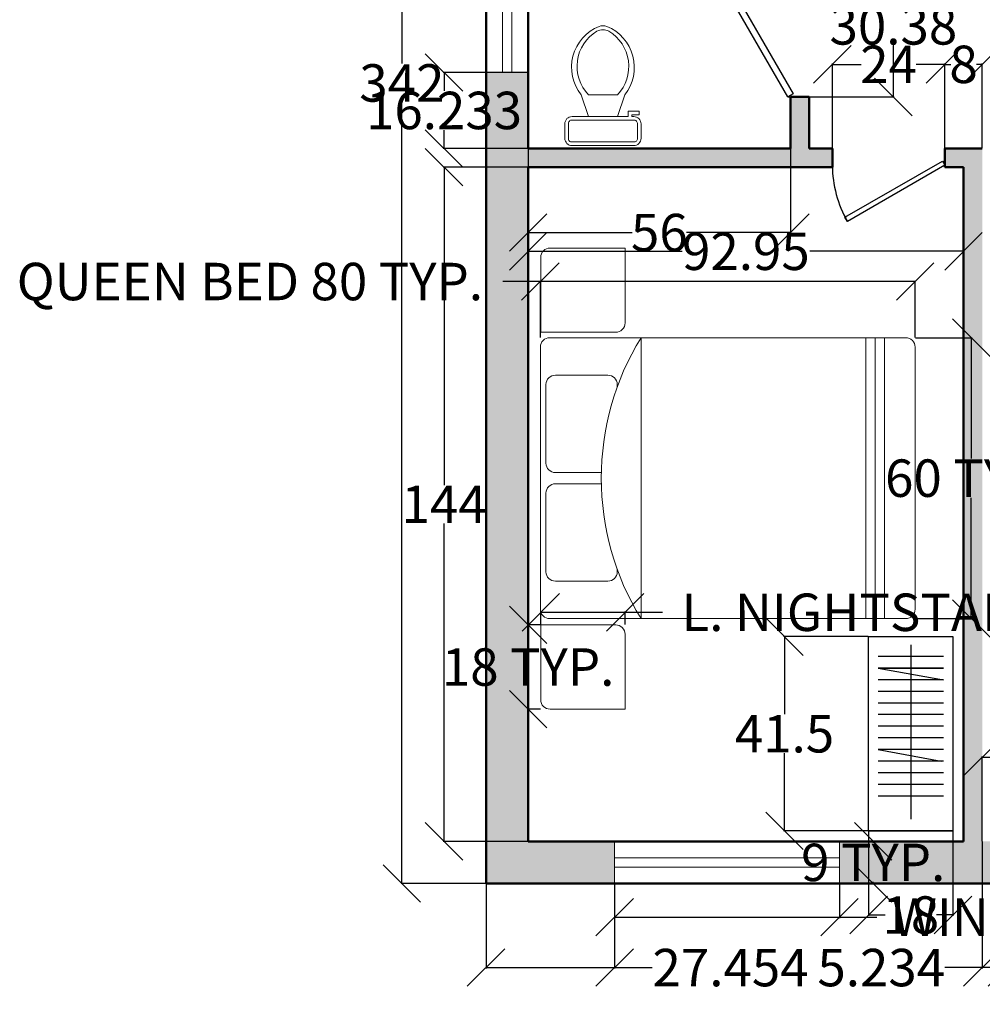
# Model space of a CAD drawing. Units: inches. Extents: x -87 to 308, y -349 to 42.
# Tile 1 of 6: x -87 to 119, y -349 to -139. Entities that reach past the tile are written whole.
import ezdxf

# ---------------------------------------------------------------- set-up
doc = ezdxf.new("R2010")
doc.units = ezdxf.units.IN
doc.header["$MEASUREMENT"] = 0
for name, color, linetype, lineweight in [('A-ANNO-DIMS', 2, 'Continuous', 18), ('A-DOOR', 3, 'Continuous', 25), ('A-FLOR-CASE', 9, 'Continuous', 25), ('A-FLOR-FIXT', 9, 'Continuous', 18), ('A-FURN', 8, 'Continuous', 18), ('A-GLAZ', 4, 'Continuous', 18), ('A-WALL', 7, 'Continuous', 50), ('A-WALL-PATT', 251, 'Continuous', 13)]:
    doc.layers.add(name, color=color, linetype=linetype, lineweight=lineweight)
doc.styles.get("Standard").update_dxf_attribs({"font": 'arial.ttf'})
doc.dimstyles.get("Standard").update_dxf_attribs({"dimtxt": 8, "dimasz": 8, "dimexe": 0.18, "dimexo": 0.0625, "dimgap": 0.09, "dimtad": 0, "dimtih": 1, "dimtoh": 1, "dimdec": 0, "dimzin": 0, "dimdsep": 46, "dimlunit": 4, "dimtxsty": 'Standard', "dimblk": 'OBLIQUE', "dimcen": 0.09, "dimadec": 0, "dimazin": 0, "dimtfac": 1, "dimtdec": 0, "dimtofl": 0, "dimtmove": 0, "dimatfit": 3, "dimldrblk": 'OBLIQUE', "dimfxl": 1, "dimtolj": 1, "dimtzin": 0, "dimarcsym": 0})

# ---------------------------------------------------------------- blocks, each defined once
blk = doc.blocks.new('*U6')
for p, q in [((-40, 0), (-40, 6)), ((0, 0), (0, 6))]:
    blk.add_line(p, q)
blk.add_lwpolyline([(0, 0), (-34.64, -20), (-35.52, -18.48), (-0.87, 1.52)], close=True)
blk.add_arc((0, 0), 40, 180, 210)
blk = doc.blocks.new('*U7')
for p, q in [((-40, 0), (-40, 6)), ((0, 0), (0, 6))]:
    blk.add_line(p, q)
blk.add_lwpolyline([(0, 0), (-34.64, -20), (-35.52, -18.48), (-0.88, 1.52)], close=True)
blk.add_arc((0, 0), 40, 180, 210)
blk = doc.blocks.new('Toilet - top')
for p, q in [((9.5, -6), (9.5, -2)), ((-8, -8.5), (-8, -8)), ((-7, -8), (-7, -9.5)), ((-4, -8), (-6, -14)), ((4, -8), (6, -14)), ((-10, -8.5), (-8, -8.5)), ((-10, -9.5), (-10, -8.5)), ((-7, -9.5), (-10, -9.5)), ((4, -14), (-4, -14))]:
    blk.add_line(p, q)
blk.add_lwpolyline([(-7, -8), (8.5, -8, 0.414214), (10.5, -6), (10.5, -2, 0.414214), (8.5, 0), (-8.5, 0, 0.414214), (-10.5, -2), (-10.5, -6, 0.414214), (-8.5, -8), (-8, -8)], format="xyb")
for points in [[(-9.5, -2), (-9.5, -6)], [(8.5, -1), (-8.5, -1)], [(-8.5, -7), (8.5, -7)]]:
    blk.add_lwpolyline(points)
for centre, radius, start, end in [((-8.62, -1.88), 0.884, 81.8699, 188.1301), ((8.62, -1.88), 0.884, 351.8699, 98.1301), ((-8.62, -6.12), 0.884, 171.8699, 278.1301), ((8.62, -6.12), 0.884, 261.8699, 8.1301), ((3.52, -21.58), 12.17, 141.4691, 247.9714), ((4.2, -21.82), 11.33, 136.3677, 238.9468), ((-3.52, -21.58), 12.17, 292.0284, 38.5307), ((-4.2, -21.82), 11.33, 301.053, 43.6321), ((0, -27.88), 4, 245.7318, 294.2682), ((0, -29), 4, 254.8605, 285.1395)]:
    blk.add_arc(centre, radius, start, end)
blk = doc.blocks.new('Bed - Queen')
for p, q in [((2, 0), (58, 0)), ((0, -78), (0, -2)), ((10, -1.2), (26.8, -1.2)), ((33.2, -1.2), (50, -1.2)), ((60, -2), (60, -78)), ((8, -14.4), (8, -3.2)), ((28.8, -3.2), (28.8, -13.02)), ((31.2, -13.02), (31.2, -3.2)), ((52, -3.2), (52, -14.4)), ((10.58, -16.4), (10, -16.4)), ((50, -16.4), (49.42, -16.4)), ((60, -21.5), (0, -21.5)), ((0, -69.5), (60, -69.5)), ((0, -71.5), (60, -71.5)), ((0, -73.5), (60, -73.5)), ((58, -80), (2, -80))]:
    blk.add_line(p, q)
for centre, radius, start, end in [((58, -2), 2, 0, 90), ((2, -2), 2, 90, 180), ((10, -3.2), 2, 90, 180), ((26.8, -3.2), 2, 0, 90), ((33.2, -3.2), 2, 90, 180), ((50, -3.2), 2, 0, 90), ((30, -70.21), 57.21, 58.3725, 121.6275), ((10, -14.4), 2, 180, 270), ((50, -14.4), 2, 270, 0), ((2, -78), 2, 180, 270), ((58, -78), 2, 270, 0)]:
    blk.add_arc(centre, radius, start, end)
blk = doc.blocks.new('WIN-48IN')
for p, q in [((0, 5.5), (48, 5.5)), ((0, 3.5), (48, 3.5))]:
    blk.add_line(p, q)
for points in [[(0, 0), (0, 9)], [(48, 9), (48, 0)]]:
    blk.add_lwpolyline(points)
blk = doc.blocks.new('WIN-24IN')
for p, q in [((0, 5.5), (24, 5.5)), ((0, 3.5), (24, 3.5))]:
    blk.add_line(p, q)
for points in [[(0, 0), (0, 9)], [(24, 9), (24, 0)]]:
    blk.add_lwpolyline(points)
blk = doc.blocks.new('NIGHTSTAND-18IN-L')
blk.add_lwpolyline([(2, 0), (18, 0), (18, 16, 0.414214), (16, 18), (0, 18), (0, 2, 0.414214)], format="xyb", close=True)
blk = doc.blocks.new('NIGHTSTAND-18IN-R')
blk.add_lwpolyline([(0, 0), (16, 0, 0.414214), (18, 2), (18, 18), (2, 18, 0.414214), (0, 16)], format="xyb", close=True)
blk = doc.blocks.new('_Oblique')
at = {"color": 0, "linetype": 'ByBlock', "lineweight": -2}
blk.add_line((-0.5, -0.5), (0.5, 0.5), dxfattribs=at)
blk = doc.blocks.new('*D23')
at = {"layer": 'A-ANNO-DIMS', "color": 0, "lineweight": -2, "transparency": 16777216}
for p, q in [((40.22, -323.73), (40.22, -331.05)), ((88.22, -323.73), (88.22, -331.05)), ((40.22, -330.87), (88.22, -330.87)), ((88.22, -330.87), (96.22, -330.87))]:
    blk.add_line(p, q, dxfattribs=at)
at = {"layer": 'Defpoints', "color": 0, "transparency": 16777216}
for p in [(40.22, -323.67), (88.22, -323.67), (88.22, -330.87)]:
    blk.add_point(p, dxfattribs=at)
at = {"layer": 'A-ANNO-DIMS', "color": 0, "lineweight": -2, "transparency": 16777216, "xscale": 8, "yscale": 8, "zscale": 8, "rotation": 180}
blk.add_blockref('_Oblique', (40.22, -330.87), dxfattribs=at)
at = {"layer": 'A-ANNO-DIMS', "color": 0, "lineweight": -2, "transparency": 16777216, "xscale": 8, "yscale": 8, "zscale": 8}
blk.add_blockref('_Oblique', (88.22, -330.87), dxfattribs=at)
at = {"layer": 'A-ANNO-DIMS', "color": 0, "transparency": 16777216, "insert": (142.01, -330.87), "char_height": 8, "attachment_point": 5}
blk.add_mtext('\\A1;WINDOW 48 TYP.', dxfattribs=at)
blk = doc.blocks.new('*D24')
at = {"layer": 'A-ANNO-DIMS', "color": 0, "lineweight": -2, "transparency": 16777216}
for p, q in [((88.28, -314.67), (95.6, -314.67)), ((95.42, -314.67), (95.42, -314.99)), ((88.28, -323.67), (95.6, -323.67)), ((95.42, -323.67), (95.42, -323.34))]:
    blk.add_line(p, q, dxfattribs=at)
at = {"layer": 'Defpoints', "color": 0, "transparency": 16777216}
for p in [(88.22, -314.67), (95.42, -314.67), (88.22, -323.67)]:
    blk.add_point(p, dxfattribs=at)
at = {"layer": 'A-ANNO-DIMS', "color": 0, "lineweight": -2, "transparency": 16777216, "xscale": 8, "yscale": 8, "zscale": 8}
for p, rotation in [((95.42, -314.67), 90), ((95.42, -323.67), 270)]:
    blk.add_blockref('_Oblique', p, dxfattribs=dict(at, rotation=rotation))
at = {"layer": 'A-ANNO-DIMS', "color": 0, "transparency": 16777216, "insert": (95.42, -319.17), "char_height": 8, "attachment_point": 5}
blk.add_mtext('\\A1;9 TYP.', dxfattribs=at)
blk = doc.blocks.new('*D29')
at = {"layer": 'A-ANNO-DIMS', "color": 0, "lineweight": -2, "transparency": 16777216}
for p, q in [((24.37, -195.09), (16.37, -195.09)), ((24.37, -207.03), (24.37, -194.91)), ((104.37, -195.09), (24.37, -195.09)), ((104.37, -207.03), (104.37, -194.91))]:
    blk.add_line(p, q, dxfattribs=at)
at = {"layer": 'Defpoints', "color": 0, "transparency": 16777216}
for p in [(24.37, -195.09), (24.37, -207.09), (104.37, -207.09)]:
    blk.add_point(p, dxfattribs=at)
at = {"layer": 'A-ANNO-DIMS', "color": 0, "lineweight": -2, "transparency": 16777216, "xscale": 8, "yscale": 8, "zscale": 8, "rotation": 180}
blk.add_blockref('_Oblique', (24.37, -195.09), dxfattribs=at)
at = {"layer": 'A-ANNO-DIMS', "color": 0, "lineweight": -2, "transparency": 16777216, "xscale": 8, "yscale": 8, "zscale": 8}
blk.add_blockref('_Oblique', (104.37, -195.09), dxfattribs=at)
at = {"layer": 'A-ANNO-DIMS', "color": 0, "transparency": 16777216, "insert": (-37.65, -195.09), "char_height": 8, "attachment_point": 5}
blk.add_mtext('\\A1;QUEEN BED 80 TYP.', dxfattribs=at)
blk = doc.blocks.new('*D30')
at = {"layer": 'A-ANNO-DIMS', "color": 0, "lineweight": -2, "transparency": 16777216}
for p, q in [((104.43, -207.09), (116.55, -207.09)), ((116.37, -207.09), (116.37, -232.92)), ((116.37, -267.09), (116.37, -241.27)), ((104.43, -267.09), (116.55, -267.09))]:
    blk.add_line(p, q, dxfattribs=at)
at = {"layer": 'Defpoints', "color": 0, "transparency": 16777216}
for p in [(104.37, -207.09), (116.37, -207.09), (104.37, -267.09)]:
    blk.add_point(p, dxfattribs=at)
at = {"layer": 'A-ANNO-DIMS', "color": 0, "lineweight": -2, "transparency": 16777216, "xscale": 8, "yscale": 8, "zscale": 8}
for p, rotation in [((116.37, -207.09), 90), ((116.37, -267.09), 270)]:
    blk.add_blockref('_Oblique', p, dxfattribs=dict(at, rotation=rotation))
at = {"layer": 'A-ANNO-DIMS', "color": 0, "transparency": 16777216, "insert": (116.37, -237.09), "char_height": 8, "attachment_point": 5}
blk.add_mtext('\\A1;60 TYP.', dxfattribs=at)
blk = doc.blocks.new('*D33')
at = {"layer": 'A-ANNO-DIMS', "color": 0, "lineweight": -2, "transparency": 16777216}
for p, q in [((26.45, -127.5), (26.45, -129.42)), ((38.45, -127.5), (38.45, -129.42)), ((26.45, -129.24), (38.45, -129.24)), ((38.45, -129.24), (46.45, -129.24))]:
    blk.add_line(p, q, dxfattribs=at)
at = {"layer": 'Defpoints', "color": 0, "transparency": 16777216}
for p in [(26.45, -127.44), (38.45, -127.44), (38.45, -129.24)]:
    blk.add_point(p, dxfattribs=at)
at = {"layer": 'A-ANNO-DIMS', "color": 0, "lineweight": -2, "transparency": 16777216, "xscale": 8, "yscale": 8, "zscale": 8, "rotation": 180}
blk.add_blockref('_Oblique', (26.45, -129.24), dxfattribs=at)
at = {"layer": 'A-ANNO-DIMS', "color": 0, "lineweight": -2, "transparency": 16777216, "xscale": 8, "yscale": 8, "zscale": 8}
blk.add_blockref('_Oblique', (38.45, -129.24), dxfattribs=at)
at = {"layer": 'A-ANNO-DIMS', "color": 0, "transparency": 16777216, "insert": (84.15, -129.24), "char_height": 8, "attachment_point": 5}
blk.add_mtext('\\A1;BASIN 12 TYP.', dxfattribs=at)
blk = doc.blocks.new('*D35')
at = {"layer": 'A-ANNO-DIMS', "color": 0, "lineweight": -2, "transparency": 16777216}
for p, q in [((24.45, -268.37), (24.45, -265.56)), ((24.45, -265.74), (42.45, -265.74)), ((42.45, -268.37), (42.45, -265.56)), ((42.45, -265.74), (50.45, -265.74))]:
    blk.add_line(p, q, dxfattribs=at)
at = {"layer": 'Defpoints', "color": 0, "transparency": 16777216}
for p in [(42.45, -265.74), (24.45, -268.44), (42.45, -268.44)]:
    blk.add_point(p, dxfattribs=at)
at = {"layer": 'A-ANNO-DIMS', "color": 0, "lineweight": -2, "transparency": 16777216, "xscale": 8, "yscale": 8, "zscale": 8, "rotation": 180}
blk.add_blockref('_Oblique', (24.45, -265.74), dxfattribs=at)
at = {"layer": 'A-ANNO-DIMS', "color": 0, "lineweight": -2, "transparency": 16777216, "xscale": 8, "yscale": 8, "zscale": 8}
blk.add_blockref('_Oblique', (42.45, -265.74), dxfattribs=at)
at = {"layer": 'A-ANNO-DIMS', "color": 0, "transparency": 16777216, "insert": (113.92, -265.74), "char_height": 8, "attachment_point": 5}
blk.add_mtext('\\A1;L. NIGHTSTAND 18 TYP.', dxfattribs=at)
blk = doc.blocks.new('*D36')
at = {"layer": 'A-ANNO-DIMS', "color": 0, "lineweight": -2, "transparency": 16777216}
for p, q in [((24.38, -268.44), (21.57, -268.44)), ((21.75, -268.44), (21.75, -273.26)), ((21.75, -286.44), (21.75, -281.61)), ((24.38, -286.44), (21.57, -286.44))]:
    blk.add_line(p, q, dxfattribs=at)
at = {"layer": 'Defpoints', "color": 0, "transparency": 16777216}
for p in [(21.75, -268.44), (24.45, -268.44), (24.45, -286.44)]:
    blk.add_point(p, dxfattribs=at)
at = {"layer": 'A-ANNO-DIMS', "color": 0, "lineweight": -2, "transparency": 16777216, "xscale": 8, "yscale": 8, "zscale": 8}
for p, rotation in [((21.75, -268.44), 90), ((21.75, -286.44), 270)]:
    blk.add_blockref('_Oblique', p, dxfattribs=dict(at, rotation=rotation))
at = {"layer": 'A-ANNO-DIMS', "color": 0, "transparency": 16777216, "insert": (21.75, -277.44), "char_height": 8, "attachment_point": 5}
blk.add_mtext('\\A1;18 TYP.', dxfattribs=at)
blk = doc.blocks.new('*D48')
at = {"layer": 'A-ANNO-DIMS', "color": 0, "lineweight": -2, "transparency": 16777216}
for p, q in [((12.7, 18.33), (-5.38, 18.33)), ((-5.2, 18.33), (-5.2, -148.49)), ((-5.2, -323.67), (-5.2, -156.85)), ((12.7, -323.67), (-5.38, -323.67))]:
    blk.add_line(p, q, dxfattribs=at)
at = {"layer": 'Defpoints', "color": 0, "transparency": 16777216}
for p in [(-5.2, 18.33), (12.76, 18.33), (12.76, -323.67)]:
    blk.add_point(p, dxfattribs=at)
at = {"layer": 'A-ANNO-DIMS', "color": 0, "lineweight": -2, "transparency": 16777216, "xscale": 8, "yscale": 8, "zscale": 8}
for p, rotation in [((-5.2, 18.33), 90), ((-5.2, -323.67), 270)]:
    blk.add_blockref('_Oblique', p, dxfattribs=dict(at, rotation=rotation))
at = {"layer": 'A-ANNO-DIMS', "color": 0, "transparency": 16777216, "insert": (-5.2, -152.67), "char_height": 8, "attachment_point": 5}
blk.add_mtext('\\A1;342', dxfattribs=at)
blk = doc.blocks.new('*D51')
at = {"layer": 'A-ANNO-DIMS', "color": 0, "lineweight": -2, "transparency": 16777216}
for p, q in [((12.76, -323.73), (12.76, -341.81)), ((40.22, -323.73), (40.22, -341.81)), ((12.76, -341.63), (40.22, -341.63)), ((40.22, -341.63), (48.22, -341.63))]:
    blk.add_line(p, q, dxfattribs=at)
at = {"layer": 'Defpoints', "color": 0, "transparency": 16777216}
for p in [(12.76, -323.67), (40.22, -323.67), (40.22, -341.63)]:
    blk.add_point(p, dxfattribs=at)
at = {"layer": 'A-ANNO-DIMS', "color": 0, "lineweight": -2, "transparency": 16777216, "xscale": 8, "yscale": 8, "zscale": 8, "rotation": 180}
blk.add_blockref('_Oblique', (12.76, -341.63), dxfattribs=at)
at = {"layer": 'A-ANNO-DIMS', "color": 0, "lineweight": -2, "transparency": 16777216, "xscale": 8, "yscale": 8, "zscale": 8}
blk.add_blockref('_Oblique', (40.22, -341.63), dxfattribs=at)
at = {"layer": 'A-ANNO-DIMS', "color": 0, "transparency": 16777216, "insert": (64.97, -341.63), "char_height": 8, "attachment_point": 5}
blk.add_mtext('\\A1;27.454', dxfattribs=at)
blk = doc.blocks.new('*D52')
at = {"layer": 'A-ANNO-DIMS', "color": 0, "lineweight": -2, "transparency": 16777216}
for p, q in [((118.71, -314.61), (118.71, -296.52)), ((142.71, -314.61), (142.71, -296.52)), ((118.71, -296.7), (124.84, -296.7)), ((142.71, -296.7), (136.58, -296.7))]:
    blk.add_line(p, q, dxfattribs=at)
at = {"layer": 'Defpoints', "color": 0, "transparency": 16777216}
for p in [(142.71, -296.7), (118.71, -314.67), (142.71, -314.67)]:
    blk.add_point(p, dxfattribs=at)
at = {"layer": 'A-ANNO-DIMS', "color": 0, "lineweight": -2, "transparency": 16777216, "xscale": 8, "yscale": 8, "zscale": 8, "rotation": 180}
blk.add_blockref('_Oblique', (118.71, -296.7), dxfattribs=at)
at = {"layer": 'A-ANNO-DIMS', "color": 0, "lineweight": -2, "transparency": 16777216, "xscale": 8, "yscale": 8, "zscale": 8}
blk.add_blockref('_Oblique', (142.71, -296.7), dxfattribs=at)
at = {"layer": 'A-ANNO-DIMS', "color": 0, "transparency": 16777216, "insert": (130.71, -296.7), "char_height": 8, "attachment_point": 5}
blk.add_mtext('\\A1;24', dxfattribs=at)
blk = doc.blocks.new('*D56')
at = {"layer": 'A-ANNO-DIMS', "color": 0, "lineweight": -2, "transparency": 16777216}
for p, q in [((21.7, -150.44), (3.62, -150.44)), ((3.8, -150.44), (3.8, -154.37)), ((3.8, -166.67), (3.8, -162.73)), ((21.7, -166.67), (3.62, -166.67))]:
    blk.add_line(p, q, dxfattribs=at)
at = {"layer": 'Defpoints', "color": 0, "transparency": 16777216}
for p in [(3.8, -150.44), (21.76, -150.44), (21.76, -166.67)]:
    blk.add_point(p, dxfattribs=at)
at = {"layer": 'A-ANNO-DIMS', "color": 0, "lineweight": -2, "transparency": 16777216, "xscale": 8, "yscale": 8, "zscale": 8}
for p, rotation in [((3.8, -150.44), 90), ((3.8, -166.67), 270)]:
    blk.add_blockref('_Oblique', p, dxfattribs=dict(at, rotation=rotation))
at = {"layer": 'A-ANNO-DIMS', "color": 0, "transparency": 16777216, "insert": (3.8, -158.55), "char_height": 8, "attachment_point": 5}
blk.add_mtext('\\A1;16.233', dxfattribs=at)
blk = doc.blocks.new('*D62')
at = {"layer": 'A-ANNO-DIMS', "color": 0, "lineweight": -2, "transparency": 16777216}
for p, q in [((21.76, -166.73), (21.76, -184.81)), ((77.76, -166.73), (77.76, -184.81)), ((21.76, -184.63), (43.95, -184.63)), ((77.76, -184.63), (55.58, -184.63))]:
    blk.add_line(p, q, dxfattribs=at)
at = {"layer": 'Defpoints', "color": 0, "transparency": 16777216}
for p in [(21.76, -166.67), (77.76, -166.67), (21.76, -184.63)]:
    blk.add_point(p, dxfattribs=at)
at = {"layer": 'A-ANNO-DIMS', "color": 0, "lineweight": -2, "transparency": 16777216, "xscale": 8, "yscale": 8, "zscale": 8, "rotation": 180}
blk.add_blockref('_Oblique', (21.76, -184.63), dxfattribs=at)
at = {"layer": 'A-ANNO-DIMS', "color": 0, "lineweight": -2, "transparency": 16777216, "xscale": 8, "yscale": 8, "zscale": 8}
blk.add_blockref('_Oblique', (77.76, -184.63), dxfattribs=at)
at = {"layer": 'A-ANNO-DIMS', "color": 0, "transparency": 16777216, "insert": (49.76, -184.63), "char_height": 8, "attachment_point": 5}
blk.add_mtext('\\A1;56', dxfattribs=at)
blk = doc.blocks.new('*D63')
at = {"layer": 'A-ANNO-DIMS', "color": 0, "lineweight": -2, "transparency": 16777216}
for p, q in [((21.76, -170.73), (21.76, -188.81)), ((114.71, -170.73), (114.71, -188.81)), ((21.76, -188.63), (54.62, -188.63)), ((114.71, -188.63), (81.86, -188.63))]:
    blk.add_line(p, q, dxfattribs=at)
at = {"layer": 'Defpoints', "color": 0, "transparency": 16777216}
for p in [(21.76, -170.67), (114.71, -170.67), (21.76, -188.63)]:
    blk.add_point(p, dxfattribs=at)
at = {"layer": 'A-ANNO-DIMS', "color": 0, "lineweight": -2, "transparency": 16777216, "xscale": 8, "yscale": 8, "zscale": 8, "rotation": 180}
blk.add_blockref('_Oblique', (21.76, -188.63), dxfattribs=at)
at = {"layer": 'A-ANNO-DIMS', "color": 0, "lineweight": -2, "transparency": 16777216, "xscale": 8, "yscale": 8, "zscale": 8}
blk.add_blockref('_Oblique', (114.71, -188.63), dxfattribs=at)
at = {"layer": 'A-ANNO-DIMS', "color": 0, "transparency": 16777216, "insert": (68.24, -188.63), "char_height": 8, "attachment_point": 5}
blk.add_mtext('\\A1;92.95', dxfattribs=at)
blk = doc.blocks.new('*D64')
at = {"layer": 'A-ANNO-DIMS', "color": 0, "lineweight": -2, "transparency": 16777216}
for p, q in [((21.7, -170.67), (3.62, -170.67)), ((3.8, -170.67), (3.8, -238.56)), ((3.8, -314.67), (3.8, -246.77)), ((21.7, -314.67), (3.62, -314.67))]:
    blk.add_line(p, q, dxfattribs=at)
at = {"layer": 'Defpoints', "color": 0, "transparency": 16777216}
for p in [(3.8, -170.67), (21.76, -170.67), (21.76, -314.67)]:
    blk.add_point(p, dxfattribs=at)
at = {"layer": 'A-ANNO-DIMS', "color": 0, "lineweight": -2, "transparency": 16777216, "xscale": 8, "yscale": 8, "zscale": 8}
for p, rotation in [((3.8, -170.67), 90), ((3.8, -314.67), 270)]:
    blk.add_blockref('_Oblique', p, dxfattribs=dict(at, rotation=rotation))
at = {"layer": 'A-ANNO-DIMS', "color": 0, "transparency": 16777216, "insert": (3.8, -242.67), "char_height": 8, "attachment_point": 5}
blk.add_mtext('\\A1;144', dxfattribs=at)
blk = doc.blocks.new('*D70')
at = {"layer": 'A-ANNO-DIMS', "color": 0, "lineweight": -2, "transparency": 16777216}
for p, q in [((81.83, -125.29), (99.91, -125.29)), ((99.73, -125.29), (99.73, -136.3)), ((99.73, -155.67), (99.73, -144.65)), ((81.83, -155.67), (99.91, -155.67))]:
    blk.add_line(p, q, dxfattribs=at)
at = {"layer": 'Defpoints', "color": 0, "transparency": 16777216}
for p in [(81.76, -125.29), (81.76, -155.67), (99.73, -155.67)]:
    blk.add_point(p, dxfattribs=at)
at = {"layer": 'A-ANNO-DIMS', "color": 0, "lineweight": -2, "transparency": 16777216, "xscale": 8, "yscale": 8, "zscale": 8}
for p, rotation in [((99.73, -125.29), 90), ((99.73, -155.67), 270)]:
    blk.add_blockref('_Oblique', p, dxfattribs=dict(at, rotation=rotation))
at = {"layer": 'A-ANNO-DIMS', "color": 0, "transparency": 16777216, "insert": (99.73, -140.48), "char_height": 8, "attachment_point": 5}
blk.add_mtext('\\A1;30.38', dxfattribs=at)
blk = doc.blocks.new('*D72')
at = {"layer": 'A-ANNO-DIMS', "color": 0, "lineweight": -2, "transparency": 16777216}
for p, q in [((86.71, -166.61), (86.71, -148.52)), ((86.71, -148.7), (92.84, -148.7)), ((110.71, -148.7), (104.58, -148.7)), ((110.71, -166.61), (110.71, -148.52))]:
    blk.add_line(p, q, dxfattribs=at)
at = {"layer": 'Defpoints', "color": 0, "transparency": 16777216}
for p in [(110.71, -148.7), (86.71, -166.67), (110.71, -166.67)]:
    blk.add_point(p, dxfattribs=at)
at = {"layer": 'A-ANNO-DIMS', "color": 0, "lineweight": -2, "transparency": 16777216, "xscale": 8, "yscale": 8, "zscale": 8, "rotation": 180}
blk.add_blockref('_Oblique', (86.71, -148.7), dxfattribs=at)
at = {"layer": 'A-ANNO-DIMS', "color": 0, "lineweight": -2, "transparency": 16777216, "xscale": 8, "yscale": 8, "zscale": 8}
blk.add_blockref('_Oblique', (110.71, -148.7), dxfattribs=at)
at = {"layer": 'A-ANNO-DIMS', "color": 0, "transparency": 16777216, "insert": (98.71, -148.7), "char_height": 8, "attachment_point": 5}
blk.add_mtext('\\A1;24', dxfattribs=at)
blk = doc.blocks.new('*D73')
at = {"layer": 'A-ANNO-DIMS', "color": 0, "lineweight": -2, "transparency": 16777216}
for p, q in [((110.71, -166.61), (110.71, -148.52)), ((110.71, -148.7), (111.99, -148.7)), ((118.71, -148.7), (117.44, -148.7)), ((118.71, -166.61), (118.71, -148.52))]:
    blk.add_line(p, q, dxfattribs=at)
at = {"layer": 'Defpoints', "color": 0, "transparency": 16777216}
for p in [(118.71, -148.7), (110.71, -166.67), (118.71, -166.67)]:
    blk.add_point(p, dxfattribs=at)
at = {"layer": 'A-ANNO-DIMS', "color": 0, "lineweight": -2, "transparency": 16777216, "xscale": 8, "yscale": 8, "zscale": 8, "rotation": 180}
blk.add_blockref('_Oblique', (110.71, -148.7), dxfattribs=at)
at = {"layer": 'A-ANNO-DIMS', "color": 0, "lineweight": -2, "transparency": 16777216, "xscale": 8, "yscale": 8, "zscale": 8}
blk.add_blockref('_Oblique', (118.71, -148.7), dxfattribs=at)
at = {"layer": 'A-ANNO-DIMS', "color": 0, "transparency": 16777216, "insert": (114.71, -148.7), "char_height": 8, "attachment_point": 5}
blk.add_mtext('\\A1;8', dxfattribs=at)
blk = doc.blocks.new('*D83')
at = {"layer": 'A-ANNO-DIMS', "color": 0, "lineweight": -2, "transparency": 16777216}
for p, q in [((94.38, -270.94), (76.3, -270.94)), ((76.48, -270.94), (76.48, -287.51)), ((76.48, -312.44), (76.48, -295.86)), ((94.38, -312.44), (76.3, -312.44))]:
    blk.add_line(p, q, dxfattribs=at)
at = {"layer": 'Defpoints', "color": 0, "transparency": 16777216}
for p in [(76.48, -270.94), (94.45, -270.94), (94.45, -312.44)]:
    blk.add_point(p, dxfattribs=at)
at = {"layer": 'A-ANNO-DIMS', "color": 0, "lineweight": -2, "transparency": 16777216, "xscale": 8, "yscale": 8, "zscale": 8}
for p, rotation in [((76.48, -270.94), 90), ((76.48, -312.44), 270)]:
    blk.add_blockref('_Oblique', p, dxfattribs=dict(at, rotation=rotation))
at = {"layer": 'A-ANNO-DIMS', "color": 0, "transparency": 16777216, "insert": (76.48, -291.69), "char_height": 8, "attachment_point": 5}
blk.add_mtext('\\A1;41.5', dxfattribs=at)
blk = doc.blocks.new('*D84')
at = {"layer": 'A-ANNO-DIMS', "color": 0, "lineweight": -2, "transparency": 16777216}
for p, q in [((94.45, -312.5), (94.45, -330.58)), ((112.45, -312.5), (112.45, -330.58)), ((94.45, -330.4), (97.99, -330.4)), ((112.45, -330.4), (108.9, -330.4))]:
    blk.add_line(p, q, dxfattribs=at)
at = {"layer": 'Defpoints', "color": 0, "transparency": 16777216}
for p in [(94.45, -312.44), (112.45, -312.44), (94.45, -330.4)]:
    blk.add_point(p, dxfattribs=at)
at = {"layer": 'A-ANNO-DIMS', "color": 0, "lineweight": -2, "transparency": 16777216, "xscale": 8, "yscale": 8, "zscale": 8, "rotation": 180}
blk.add_blockref('_Oblique', (94.45, -330.4), dxfattribs=at)
at = {"layer": 'A-ANNO-DIMS', "color": 0, "lineweight": -2, "transparency": 16777216, "xscale": 8, "yscale": 8, "zscale": 8}
blk.add_blockref('_Oblique', (112.45, -330.4), dxfattribs=at)
at = {"layer": 'A-ANNO-DIMS', "color": 0, "transparency": 16777216, "insert": (103.45, -330.4), "char_height": 8, "attachment_point": 5}
blk.add_mtext('\\A1;18', dxfattribs=at)
blk = doc.blocks.new('*D90')
at = {"layer": 'A-ANNO-DIMS', "color": 0, "lineweight": -2, "transparency": 16777216}
for p, q in [((123.95, -291), (123.95, -341.81)), ((118.71, -314.73), (118.71, -341.81)), ((118.71, -341.63), (110.71, -341.63)), ((123.95, -341.63), (118.71, -341.63))]:
    blk.add_line(p, q, dxfattribs=at)
at = {"layer": 'Defpoints', "color": 0, "transparency": 16777216}
for p in [(123.95, -290.94), (118.71, -314.67), (118.71, -341.63)]:
    blk.add_point(p, dxfattribs=at)
at = {"layer": 'A-ANNO-DIMS', "color": 0, "lineweight": -2, "transparency": 16777216, "xscale": 8, "yscale": 8, "zscale": 8, "rotation": 180}
blk.add_blockref('_Oblique', (118.71, -341.63), dxfattribs=at)
at = {"layer": 'A-ANNO-DIMS', "color": 0, "lineweight": -2, "transparency": 16777216, "xscale": 8, "yscale": 8, "zscale": 8}
blk.add_blockref('_Oblique', (123.95, -341.63), dxfattribs=at)
at = {"layer": 'A-ANNO-DIMS', "color": 0, "transparency": 16777216, "insert": (97.14, -341.63), "char_height": 8, "attachment_point": 5}
blk.add_mtext('\\A1;5.234', dxfattribs=at)

msp = doc.modelspace()

# ---------------------------------------------------------------- hatches: boundary and pattern name
at = {"layer": 'A-WALL-PATT'}
h = msp.add_hatch(color=256, dxfattribs=at)
h.dxf.hatch_style = 1
h.paths.add_polyline_path([(21.7637, -170.668), (86.7127, -170.668), (86.7127, -166.668), (81.7637, -166.668), (81.7637, -155.668), (77.7637, -155.668), (77.7637, -166.668), (21.7637, -166.668), (21.7637, -150.4351), (12.7637, -150.4351), (12.7637, -323.668), (40.2177, -323.668), (40.2177, -314.668), (21.7637, -314.668)])
h = msp.add_hatch(color=256, dxfattribs=at)
h.dxf.hatch_style = 1
h.paths.add_polyline_path([(118.7127, -170.668), (118.7127, -166.668), (114.7127, -166.668), (110.7127, -166.668), (110.7127, -170.668), (114.7127, -170.668), (114.7127, -314.668), (88.2177, -314.668), (88.2177, -323.668), (142.7127, -323.668), (142.7127, -319.1107), (142.7127, -314.668), (118.7127, -314.668)])

# ---------------------------------------------------------------- linework, layer by layer
at = {"layer": 'A-FLOR-CASE'}
for p, q in [((94.4465, -270.9351), (112.4465, -270.9351)), ((103.4465, -272.711), (103.4465, -309.9524)), ((110.4465, -275.1937), (96.4465, -275.1937)), ((110.4465, -282.642), (96.4465, -282.642)), ((110.4465, -285.1248), (96.4465, -285.1248)), ((110.4465, -287.6075), (96.4465, -287.6075)), ((110.4465, -290.0903), (96.4465, -290.0903)), ((110.4465, -292.573), (96.4465, -292.573)), ((110.4465, -297.5386), (96.4465, -297.5386)), ((110.4465, -300.0213), (96.4465, -300.0213)), ((110.4465, -302.5041), (96.4465, -302.5041)), ((110.4465, -304.9868), (96.4465, -304.9868))]:
    msp.add_line(p, q, dxfattribs=at)
for points in [[(94.4465, -312.4351), (94.4465, -270.9351)], [(112.4465, -270.9351), (112.4465, -312.4351), (94.4465, -312.4351), (112.4465, -312.4351)], [(96.4465, -277.6765), (110.4465, -277.6765), (96.4465, -277.6765), (110.4465, -280.1593), (96.4465, -280.1593)], [(110.4465, -295.0558), (96.4465, -295.0558), (109.9465, -297.5386)]]:
    msp.add_lwpolyline(points, dxfattribs=at)
at = {"layer": 'A-WALL'}
for p, q in [((21.7637, -166.668), (21.7637, -114.668)), ((77.7637, -166.668), (77.7637, -155.668)), ((81.7637, -155.668), (77.7637, -155.668)), ((81.7637, -166.668), (81.7637, -155.668)), ((77.7637, -166.668), (21.7637, -166.668)), ((86.7127, -166.668), (81.7637, -166.668)), ((86.7127, -170.668), (86.7127, -166.668)), ((114.7127, -166.668), (110.7127, -166.668)), ((110.7127, -170.668), (110.7127, -166.668)), ((114.7127, -166.668), (118.7127, -166.668)), ((21.7637, -314.668), (21.7637, -170.668)), ((86.7127, -170.668), (21.7637, -170.668)), ((114.7127, -170.668), (110.7127, -170.668)), ((114.7127, -170.668), (114.7127, -314.668)), ((114.7127, -314.668), (21.7637, -314.668))]:
    msp.add_line(p, q, dxfattribs=at)
msp.add_lwpolyline([(142.7127, -323.668), (12.7637, -323.668), (12.7637, 18.332), (246.7637, 18.332), (246.7637, -323.668), (172.7127, -323.668)], dxfattribs=at)

# ---------------------------------------------------------------- block references
at = {"layer": 'A-DOOR', "xscale": 0.7595575434647344, "yscale": 0.7595575434647344, "zscale": 0.7595575434647344, "rotation": 270}
msp.add_blockref('*U6', (77.2063, -155.668), dxfattribs=at)
at = {"layer": 'A-DOOR', "xscale": 0.6, "yscale": 0.6, "zscale": 0.6}
msp.add_blockref('*U7', (110.7127, -170.268), dxfattribs=at)
at = {"layer": 'A-FLOR-FIXT', "xscale": 0.7748713842371889, "yscale": 0.7748713842371889, "zscale": 0.7748713842371889, "rotation": 180}
msp.add_blockref('Toilet - top', (37.7161, -166.0445), dxfattribs=at)
at = {"layer": 'A-FURN'}
for name, p in [('NIGHTSTAND-18IN-R', (24.447, -205.935)), ('NIGHTSTAND-18IN-L', (24.447, -286.435))]:
    msp.add_blockref(name, p, dxfattribs=at)
at = {"layer": 'A-FURN', "rotation": 90}
msp.add_blockref('Bed - Queen', (24.3666, -267.0911), dxfattribs=at)
at = {"layer": 'A-GLAZ', "rotation": 270}
msp.add_blockref('WIN-24IN', (12.7637, -126.4351), dxfattribs=at)
at = {"layer": 'A-GLAZ'}
msp.add_blockref('WIN-48IN', (40.2176, -323.668), dxfattribs=at)

# ---------------------------------------------------------------- dimensions: what is measured, and where the dimension line sits
at = {"layer": 'A-ANNO-DIMS'}
for base, p1, p2, angle, override, picture, middle in [((-5.2008, 18.332), (12.7637, -323.668), (12.7637, 18.332), 90, {"dimdec": 0, "dimlfac": 1, "dimrnd": 0, "dimzin": 0, "dimdsep": 46, "dimlunit": 2}, '*D48', (-5.2008, -152.668)), ((99.7282, -155.668), (81.7637, -125.2857), (81.7637, -155.668), 270, {"dimdec": 2, "dimlfac": 1, "dimrnd": 0, "dimzin": 0, "dimdsep": 46, "dimlunit": 2}, '*D70', (99.7282, -140.4769)), ((118.7127, -148.7035), (110.7127, -166.668), (118.7127, -166.668), 0, {"dimdec": 0, "dimlfac": 1, "dimrnd": 0, "dimzin": 0, "dimdsep": 46, "dimlunit": 2}, '*D73', (114.7127, -148.7035)), ((3.7992, -150.4351), (21.7637, -166.668), (21.7637, -150.4351), 90, {"dimdec": 3, "dimlfac": 1, "dimrnd": 0, "dimzin": 0, "dimdsep": 46, "dimlunit": 2}, '*D56', (3.7992, -158.5516)), ((3.7992, -170.668), (21.7637, -314.668), (21.7637, -170.668), 90, {"dimdec": 0, "dimlfac": 1, "dimrnd": 0, "dimzin": 0, "dimdsep": 46, "dimlunit": 2}, '*D64', (3.7992, -242.668)), ((21.7637, -184.6325), (77.7637, -166.668), (21.7637, -166.668), 180, {"dimdec": 0, "dimlfac": 1, "dimrnd": 0, "dimzin": 0, "dimdsep": 46, "dimlunit": 2}, '*D62', (49.7637, -184.6325)), ((21.7637, -188.6325), (114.7127, -170.668), (21.7637, -170.668), 180, {"dimdec": 2, "dimlfac": 1, "dimrnd": 0, "dimzin": 0, "dimdsep": 46, "dimlunit": 2}, '*D63', (68.2382, -188.6325)), ((76.482, -270.9351), (94.4465, -312.4351), (94.4465, -270.9351), 90, {"dimdec": 1, "dimlfac": 1, "dimrnd": 0, "dimzin": 0, "dimdsep": 46, "dimlunit": 2}, '*D83', (76.482, -291.6851)), ((94.4465, -330.3996), (112.4465, -312.4351), (94.4465, -312.4351), 180, {"dimdec": 0, "dimlfac": 1, "dimrnd": 0, "dimzin": 0, "dimdsep": 46, "dimlunit": 2}, '*D84', (103.4465, -330.3996))]:
    dim = msp.add_linear_dim(base=base, p1=p1, p2=p2, angle=angle, dimstyle='Standard', override=override, dxfattribs=at)
    dim.commit()
    dim.dimension.update_dxf_attribs({"geometry": picture, "text_midpoint": middle})
for base, p1, p2, text, picture, middle in [((38.4465, -129.2351), (26.4465, -127.4351), (38.4465, -127.4351), 'BASIN <> TYP.', '*D33', (84.1518, -129.2351)), ((42.4465, -265.7351), (24.4465, -268.4351), (42.4465, -268.4351), 'L. NIGHTSTAND <> TYP.', '*D35', (113.9171, -265.7351)), ((88.2177, -330.868), (40.2177, -323.668), (88.2177, -323.668), 'WINDOW <> TYP.', '*D23', (142.013, -330.868))]:
    dim = msp.add_linear_dim(base=base, p1=p1, p2=p2, text=text, dimstyle='Standard', override={"dimdec": 0, "dimlfac": 1, "dimrnd": 0, "dimzin": 0, "dimdsep": 46, "dimlunit": 2}, dxfattribs=at)
    dim.commit()
    dim.dimension.update_dxf_attribs({"geometry": picture, "text_midpoint": middle})
for base, p1, p2, override, picture, middle in [((110.7127, -148.7035), (86.7127, -166.668), (110.7127, -166.668), {"dimdec": 0, "dimlfac": 1, "dimrnd": 0, "dimzin": 0, "dimdsep": 46, "dimlunit": 2}, '*D72', (98.7127, -148.7035)), ((118.7127, -341.6325), (123.9465, -290.9351), (118.7127, -314.668), {"dimdec": 3, "dimlfac": 1, "dimrnd": 0, "dimzin": 0, "dimdsep": 46, "dimlunit": 2}, '*D90', (97.1411, -341.6325)), ((142.7127, -296.7035), (118.7127, -314.668), (142.7127, -314.668), {"dimdec": 0, "dimlfac": 1, "dimrnd": 0, "dimzin": 0, "dimdsep": 46, "dimlunit": 2}, '*D52', (130.7127, -296.7035)), ((40.2177, -341.6325), (12.7637, -323.668), (40.2177, -323.668), {"dimdec": 3, "dimlfac": 1, "dimrnd": 0, "dimzin": 0, "dimdsep": 46, "dimlunit": 2}, '*D51', (64.9652, -341.6325))]:
    dim = msp.add_linear_dim(base=base, p1=p1, p2=p2, dimstyle='Standard', override=override, dxfattribs=at)
    dim.commit()
    dim.dimension.update_dxf_attribs({"geometry": picture, "text_midpoint": middle})
for base, p1, p2, angle, text, picture, middle in [((24.3666, -195.0911), (104.3666, -207.0911), (24.3666, -207.0911), 180, 'QUEEN BED <> TYP.', '*D29', (-37.6525, -195.0911)), ((116.3666, -207.0911), (104.3666, -267.0911), (104.3666, -207.0911), 90, '<> TYP.', '*D30', (116.3666, -237.0911)), ((21.7465, -268.4351), (24.4465, -286.4351), (24.4465, -268.4351), 90, '<> TYP.', '*D36', (21.7465, -277.4351)), ((95.4177, -314.668), (88.2177, -323.668), (88.2177, -314.668), 90, '<> TYP.', '*D24', (95.4177, -319.168))]:
    dim = msp.add_linear_dim(base=base, p1=p1, p2=p2, angle=angle, text=text, dimstyle='Standard', override={"dimdec": 0, "dimlfac": 1, "dimrnd": 0, "dimzin": 0, "dimdsep": 46, "dimlunit": 2}, dxfattribs=at)
    dim.commit()
    dim.dimension.update_dxf_attribs({"geometry": picture, "text_midpoint": middle})

doc.saveas('drawing.dxf')
